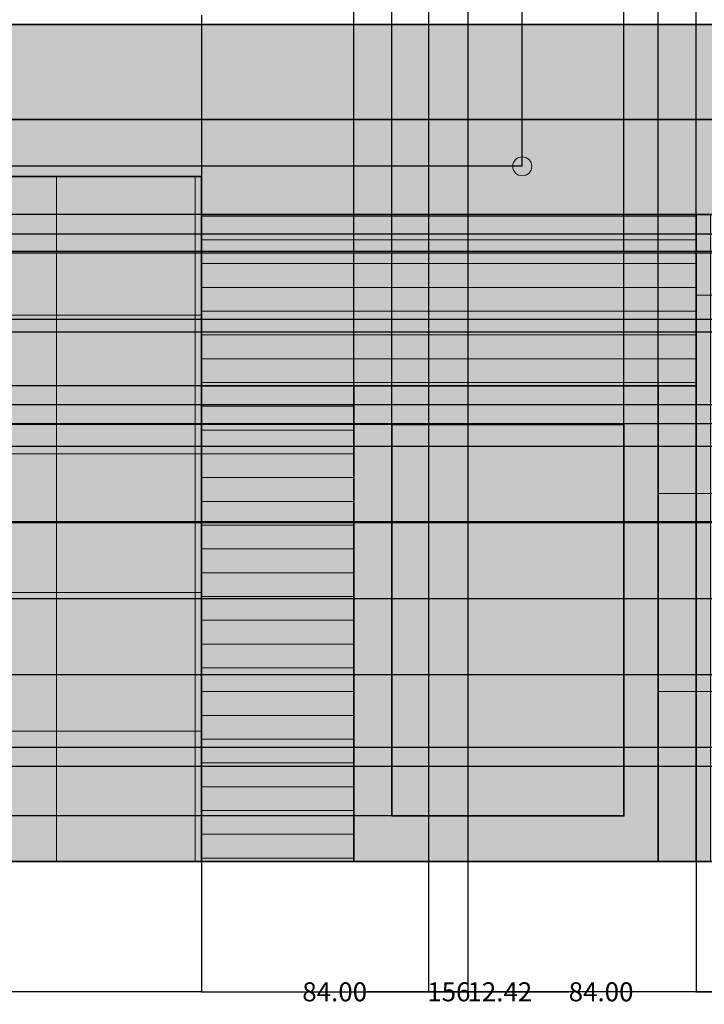
# Model space of a CAD drawing. Units: inches. Extents: x 148 to 1080, y 89 to 707.
# Tile 7 of 12: x 470 to 686, y 89 to 399. Entities that reach past the tile are written whole.
import ezdxf

# ---------------------------------------------------------------- set-up
doc = ezdxf.new("R2010")
doc.units = ezdxf.units.IN
doc.header["$MEASUREMENT"] = 0
for name, color, linetype, lineweight in [('A-ANNO-DIMS', 2, 'Continuous', 18), ('A-ELEV', 7, 'Continuous', 35), ('A-ELEV-PATT', 8, 'Continuous', 13), ('E-LITE', 3, 'Continuous', 18)]:
    doc.layers.add(name, color=color, linetype=linetype, lineweight=lineweight)
doc.styles.get("Standard").update_dxf_attribs({"font": 'arial.ttf'})
doc.dimstyles.get("Standard").update_dxf_attribs({"dimtxt": 6, "dimasz": 0.18, "dimexe": 0.18, "dimexo": 0.0625, "dimgap": 0.09, "dimtad": 0, "dimtih": 1, "dimtoh": 1, "dimdec": 0, "dimzin": 0, "dimdsep": 46, "dimlunit": 3, "dimtxsty": 'Standard', "dimcen": 0.09, "dimadec": 0, "dimazin": 0, "dimtfac": 1, "dimtdec": 0, "dimtofl": 0, "dimtmove": 0, "dimatfit": 3, "dimfxl": 1, "dimtolj": 1, "dimtzin": 0, "dimarcsym": 0})

# ---------------------------------------------------------------- blocks, each defined once
blk = doc.blocks.new('*D1')
at = {"layer": 'A-ANNO-DIMS', "color": 0, "lineweight": -2, "transparency": 16777216}
for p, q in [((215.02, 662.01), (215.02, 703.28)), ((215.2, 703.1), (604.32, 703.1)), ((1006.77, 703.1), (617.65, 703.1)), ((1006.95, 338.01), (1006.95, 703.28))]:
    blk.add_line(p, q, dxfattribs=at)
at = {"layer": 'A-ANNO-DIMS', "color": 0, "transparency": 16777216}
for points in [[(215.2, 703.13), (215.2, 703.07), (215.02, 703.1)], [(1006.77, 703.13), (1006.77, 703.07), (1006.95, 703.1)]]:
    blk.add_solid(points, dxfattribs=at)
at = {"layer": 'Defpoints', "color": 0, "transparency": 16777216}
for p in [(1006.95, 703.1), (215.02, 661.95), (1006.95, 337.95)]:
    blk.add_point(p, dxfattribs=at)
at = {"layer": 'A-ANNO-DIMS', "color": 0, "transparency": 16777216, "insert": (610.98, 703.1), "char_height": 6, "attachment_point": 5}
blk.add_mtext('\\A1;792', dxfattribs=at)
blk = doc.blocks.new('*D2')
at = {"layer": 'A-ANNO-DIMS', "color": 0, "lineweight": -2, "transparency": 16777216}
for p, q in [((251.02, 133.88), (251.02, 92.62)), ((527.02, 133.88), (527.02, 92.62)), ((251.2, 92.8), (382.25, 92.8)), ((526.84, 92.8), (395.79, 92.8))]:
    blk.add_line(p, q, dxfattribs=at)
at = {"layer": 'A-ANNO-DIMS', "color": 0, "transparency": 16777216}
for points in [[(251.2, 92.83), (251.2, 92.77), (251.02, 92.8)], [(526.84, 92.83), (526.84, 92.77), (527.02, 92.8)]]:
    blk.add_solid(points, dxfattribs=at)
at = {"layer": 'Defpoints', "color": 0, "transparency": 16777216}
for p in [(251.02, 133.95), (527.02, 133.95), (527.02, 92.8)]:
    blk.add_point(p, dxfattribs=at)
at = {"layer": 'A-ANNO-DIMS', "color": 0, "transparency": 16777216, "insert": (389.02, 92.8), "char_height": 6, "attachment_point": 5}
blk.add_mtext('\\A1;276', dxfattribs=at)
blk = doc.blocks.new('*D3')
at = {"layer": 'A-ANNO-DIMS', "color": 0, "lineweight": -2, "transparency": 16777216}
for p, q in [((527.02, 133.88), (527.02, 92.62)), ((683.02, 133.88), (683.02, 92.62)), ((527.2, 92.8), (598.59, 92.8)), ((682.84, 92.8), (611.45, 92.8))]:
    blk.add_line(p, q, dxfattribs=at)
at = {"layer": 'A-ANNO-DIMS', "color": 0, "transparency": 16777216}
for points in [[(527.2, 92.83), (527.2, 92.77), (527.02, 92.8)], [(682.84, 92.83), (682.84, 92.77), (683.02, 92.8)]]:
    blk.add_solid(points, dxfattribs=at)
at = {"layer": 'Defpoints', "color": 0, "transparency": 16777216}
for p in [(527.02, 133.95), (683.02, 133.95), (683.02, 92.8)]:
    blk.add_point(p, dxfattribs=at)
at = {"layer": 'A-ANNO-DIMS', "color": 0, "transparency": 16777216, "insert": (605.02, 92.8), "char_height": 6, "attachment_point": 5}
blk.add_mtext('\\A1;156', dxfattribs=at)
blk = doc.blocks.new('*D4')
at = {"layer": 'A-ANNO-DIMS', "color": 0, "lineweight": -2, "transparency": 16777216}
for p, q in [((683.02, 133.88), (683.02, 92.62)), ((719.02, 133.88), (719.02, 92.62)), ((683.2, 92.8), (696.64, 92.8)), ((718.84, 92.8), (705.4, 92.8))]:
    blk.add_line(p, q, dxfattribs=at)
at = {"layer": 'A-ANNO-DIMS', "color": 0, "transparency": 16777216}
for points in [[(683.2, 92.83), (683.2, 92.77), (683.02, 92.8)], [(718.84, 92.83), (718.84, 92.77), (719.02, 92.8)]]:
    blk.add_solid(points, dxfattribs=at)
at = {"layer": 'Defpoints', "color": 0, "transparency": 16777216}
for p in [(683.02, 133.95), (719.02, 133.95), (719.02, 92.8)]:
    blk.add_point(p, dxfattribs=at)
at = {"layer": 'A-ANNO-DIMS', "color": 0, "transparency": 16777216, "insert": (701.02, 92.8), "char_height": 6, "attachment_point": 5}
blk.add_mtext('\\A1;36', dxfattribs=at)
blk = doc.blocks.new('*D18')
at = {"layer": 'A-ANNO-DIMS', "color": 0, "lineweight": -2, "transparency": 16777216}
for p, q in [((635.08, 661.95), (1064.5, 661.95)), ((1064.32, 661.77), (1064.32, 401.1)), ((1064.32, 134.13), (1064.32, 394.79)), ((1007.01, 133.95), (1064.5, 133.95))]:
    blk.add_line(p, q, dxfattribs=at)
at = {"layer": 'A-ANNO-DIMS', "color": 0, "transparency": 16777216}
for points in [[(1064.29, 661.77), (1064.35, 661.77), (1064.32, 661.95)], [(1064.29, 134.13), (1064.35, 134.13), (1064.32, 133.95)]]:
    blk.add_solid(points, dxfattribs=at)
at = {"layer": 'Defpoints', "color": 0, "transparency": 16777216}
for p in [(635.02, 661.95), (1064.32, 661.95), (1006.95, 133.95)]:
    blk.add_point(p, dxfattribs=at)
at = {"layer": 'A-ANNO-DIMS', "color": 0, "transparency": 16777216, "insert": (1064.32, 397.95), "char_height": 6, "attachment_point": 5}
blk.add_mtext('\\A1;528', dxfattribs=at)
blk = doc.blocks.new('*D31')
at = {"layer": 'A-ANNO-DIMS', "color": 0, "lineweight": -2, "transparency": 16777216}
for p, q in [((587.06, 271.84), (587.06, 703.28)), ((587.24, 703.1), (613.42, 703.1)), ((660.03, 703.1), (633.85, 703.1)), ((660.21, 271.84), (660.21, 703.28))]:
    blk.add_line(p, q, dxfattribs=at)
at = {"layer": 'A-ANNO-DIMS', "color": 0, "transparency": 16777216}
for points in [[(587.24, 703.13), (587.24, 703.07), (587.06, 703.1)], [(660.03, 703.13), (660.03, 703.07), (660.21, 703.1)]]:
    blk.add_solid(points, dxfattribs=at)
at = {"layer": 'Defpoints', "color": 0, "transparency": 16777216}
for p in [(660.21, 703.1), (587.06, 271.77), (660.21, 271.77)]:
    blk.add_point(p, dxfattribs=at)
at = {"layer": 'A-ANNO-DIMS', "color": 0, "transparency": 16777216, "insert": (623.64, 703.1), "char_height": 6, "attachment_point": 5}
blk.add_mtext('\\A1;73.15', dxfattribs=at)
blk = doc.blocks.new('*D32')
at = {"layer": 'A-ANNO-DIMS', "color": 0, "lineweight": -2, "transparency": 16777216}
for p, q in [((587, 271.77), (160.42, 271.77)), ((160.6, 271.59), (160.6, 213.18)), ((160.6, 148.46), (160.6, 206.87)), ((587, 148.28), (160.42, 148.28))]:
    blk.add_line(p, q, dxfattribs=at)
at = {"layer": 'A-ANNO-DIMS', "color": 0, "transparency": 16777216}
for points in [[(160.57, 271.59), (160.63, 271.59), (160.6, 271.77)], [(160.57, 148.46), (160.63, 148.46), (160.6, 148.28)]]:
    blk.add_solid(points, dxfattribs=at)
at = {"layer": 'Defpoints', "color": 0, "transparency": 16777216}
for p in [(160.6, 271.77), (587.06, 271.77), (587.06, 148.28)]:
    blk.add_point(p, dxfattribs=at)
at = {"layer": 'A-ANNO-DIMS', "color": 0, "transparency": 16777216, "insert": (160.6, 210.03), "char_height": 6, "attachment_point": 5}
blk.add_mtext('\\A1;123.5', dxfattribs=at)
blk = doc.blocks.new('*D33')
at = {"layer": 'A-ANNO-DIMS', "color": 0, "lineweight": -2, "transparency": 16777216}
for p, q in [((575.02, 284.01), (575.02, 703.28)), ((575.2, 703.1), (618.63, 703.1)), ((670.84, 703.1), (627.41, 703.1)), ((671.02, 284.01), (671.02, 703.28))]:
    blk.add_line(p, q, dxfattribs=at)
at = {"layer": 'A-ANNO-DIMS', "color": 0, "transparency": 16777216}
for points in [[(575.2, 703.13), (575.2, 703.07), (575.02, 703.1)], [(670.84, 703.13), (670.84, 703.07), (671.02, 703.1)]]:
    blk.add_solid(points, dxfattribs=at)
at = {"layer": 'Defpoints', "color": 0, "transparency": 16777216}
for p in [(671.02, 703.1), (575.02, 283.95), (671.02, 283.95)]:
    blk.add_point(p, dxfattribs=at)
at = {"layer": 'A-ANNO-DIMS', "color": 0, "transparency": 16777216, "insert": (623.02, 703.1), "char_height": 6, "attachment_point": 5}
blk.add_mtext('\\A1;96', dxfattribs=at)
blk = doc.blocks.new('*D34')
at = {"layer": 'A-ANNO-DIMS', "color": 0, "lineweight": -2, "transparency": 16777216}
for p, q in [((574.96, 283.95), (160.42, 283.95)), ((160.6, 283.77), (160.6, 212.1)), ((160.6, 134.13), (160.6, 205.79)), ((574.96, 133.95), (160.42, 133.95))]:
    blk.add_line(p, q, dxfattribs=at)
at = {"layer": 'A-ANNO-DIMS', "color": 0, "transparency": 16777216}
for points in [[(160.57, 283.77), (160.63, 283.77), (160.6, 283.95)], [(160.57, 134.13), (160.63, 134.13), (160.6, 133.95)]]:
    blk.add_solid(points, dxfattribs=at)
at = {"layer": 'Defpoints', "color": 0, "transparency": 16777216}
for p in [(575.02, 283.95), (160.6, 133.95), (575.02, 133.95)]:
    blk.add_point(p, dxfattribs=at)
at = {"layer": 'A-ANNO-DIMS', "color": 0, "transparency": 16777216, "insert": (160.6, 208.95), "char_height": 6, "attachment_point": 5}
blk.add_mtext('\\A1;150', dxfattribs=at)
blk = doc.blocks.new('*D38')
at = {"layer": 'A-ANNO-DIMS', "color": 0, "lineweight": -2, "transparency": 16777216}
for p, q in [((934.89, 271.95), (160.42, 271.95)), ((160.6, 271.77), (160.6, 206.1)), ((160.6, 134.13), (160.6, 199.79)), ((934.89, 133.95), (160.42, 133.95))]:
    blk.add_line(p, q, dxfattribs=at)
at = {"layer": 'A-ANNO-DIMS', "color": 0, "transparency": 16777216}
for points in [[(160.57, 271.77), (160.63, 271.77), (160.6, 271.95)], [(160.57, 134.13), (160.63, 134.13), (160.6, 133.95)]]:
    blk.add_solid(points, dxfattribs=at)
at = {"layer": 'Defpoints', "color": 0, "transparency": 16777216}
for p in [(934.95, 271.95), (160.6, 133.95), (934.95, 133.95)]:
    blk.add_point(p, dxfattribs=at)
at = {"layer": 'A-ANNO-DIMS', "color": 0, "transparency": 16777216, "insert": (160.6, 202.95), "char_height": 6, "attachment_point": 5}
blk.add_mtext('\\A1;138', dxfattribs=at)
blk = doc.blocks.new('*D39')
at = {"layer": 'A-ANNO-DIMS', "color": 0, "lineweight": -2, "transparency": 16777216}
for p, q in [((946.89, 337.95), (160.42, 337.95)), ((160.6, 337.77), (160.6, 311.1)), ((160.6, 278.13), (160.6, 304.79)), ((946.89, 277.95), (160.42, 277.95))]:
    blk.add_line(p, q, dxfattribs=at)
at = {"layer": 'A-ANNO-DIMS', "color": 0, "transparency": 16777216}
for points in [[(160.57, 337.77), (160.63, 337.77), (160.6, 337.95)], [(160.57, 278.13), (160.63, 278.13), (160.6, 277.95)]]:
    blk.add_solid(points, dxfattribs=at)
at = {"layer": 'Defpoints', "color": 0, "transparency": 16777216}
for p in [(160.6, 337.95), (946.95, 337.95), (946.95, 277.95)]:
    blk.add_point(p, dxfattribs=at)
at = {"layer": 'A-ANNO-DIMS', "color": 0, "transparency": 16777216, "insert": (160.6, 307.95), "char_height": 6, "attachment_point": 5}
blk.add_mtext('\\A1;60', dxfattribs=at)
blk = doc.blocks.new('*D42')
at = {"layer": 'A-ANNO-DIMS', "color": 0, "lineweight": -2, "transparency": 16777216}
for p, q in [((772.96, 367.95), (160.42, 367.95)), ((160.6, 367.77), (160.6, 350.31)), ((160.6, 326.54), (160.6, 344)), ((718.96, 326.36), (160.42, 326.36))]:
    blk.add_line(p, q, dxfattribs=at)
at = {"layer": 'A-ANNO-DIMS', "color": 0, "transparency": 16777216}
for points in [[(160.57, 367.77), (160.63, 367.77), (160.6, 367.95)], [(160.57, 326.54), (160.63, 326.54), (160.6, 326.36)]]:
    blk.add_solid(points, dxfattribs=at)
at = {"layer": 'Defpoints', "color": 0, "transparency": 16777216}
for p in [(773.02, 367.95), (160.6, 326.36), (719.02, 326.36)]:
    blk.add_point(p, dxfattribs=at)
at = {"layer": 'A-ANNO-DIMS', "color": 0, "transparency": 16777216, "insert": (160.6, 347.16), "char_height": 6, "attachment_point": 5}
blk.add_mtext('\\A1;41.584', dxfattribs=at)
blk = doc.blocks.new('*D43')
at = {"layer": 'A-ANNO-DIMS', "color": 0, "lineweight": -2, "transparency": 16777216}
for p, q in [((765.88, 241.1), (160.42, 241.1)), ((160.6, 240.92), (160.6, 190.68)), ((160.6, 134.13), (160.6, 184.37)), ((776.65, 133.95), (160.42, 133.95))]:
    blk.add_line(p, q, dxfattribs=at)
at = {"layer": 'A-ANNO-DIMS', "color": 0, "transparency": 16777216}
for points in [[(160.57, 240.92), (160.63, 240.92), (160.6, 241.1)], [(160.57, 134.13), (160.63, 134.13), (160.6, 133.95)]]:
    blk.add_solid(points, dxfattribs=at)
at = {"layer": 'Defpoints', "color": 0, "transparency": 16777216}
for p in [(765.95, 241.1), (160.6, 133.95), (776.71, 133.95)]:
    blk.add_point(p, dxfattribs=at)
at = {"layer": 'A-ANNO-DIMS', "color": 0, "transparency": 16777216, "insert": (160.6, 187.52), "char_height": 6, "attachment_point": 5}
blk.add_mtext('\\A1;107.15', dxfattribs=at)
blk = doc.blocks.new('*D47')
at = {"layer": 'A-ANNO-DIMS', "color": 0, "lineweight": -2, "transparency": 16777216}
for p, q in [((628.17, 353.26), (628.17, 703.28)), ((628.35, 703.1), (645.36, 703.1)), ((682.84, 703.1), (665.83, 703.1)), ((683.02, 338.01), (683.02, 703.28))]:
    blk.add_line(p, q, dxfattribs=at)
at = {"layer": 'A-ANNO-DIMS', "color": 0, "transparency": 16777216}
for points in [[(628.35, 703.13), (628.35, 703.07), (628.17, 703.1)], [(682.84, 703.13), (682.84, 703.07), (683.02, 703.1)]]:
    blk.add_solid(points, dxfattribs=at)
at = {"layer": 'Defpoints', "color": 0, "transparency": 16777216}
for p in [(683.02, 703.1), (628.17, 353.2), (683.02, 337.95)]:
    blk.add_point(p, dxfattribs=at)
at = {"layer": 'A-ANNO-DIMS', "color": 0, "transparency": 16777216, "insert": (655.6, 703.1), "char_height": 6, "attachment_point": 5}
blk.add_mtext('\\A1;54.85', dxfattribs=at)
blk = doc.blocks.new('*D48')
at = {"layer": 'A-ANNO-DIMS', "color": 0, "lineweight": -2, "transparency": 16777216}
for p, q in [((683.02, 338.01), (683.02, 703.28)), ((683.2, 703.1), (694.68, 703.1)), ((726.76, 703.1), (715.28, 703.1)), ((726.94, 354.92), (726.94, 703.28))]:
    blk.add_line(p, q, dxfattribs=at)
at = {"layer": 'A-ANNO-DIMS', "color": 0, "transparency": 16777216}
for points in [[(683.2, 703.13), (683.2, 703.07), (683.02, 703.1)], [(726.76, 703.13), (726.76, 703.07), (726.94, 703.1)]]:
    blk.add_solid(points, dxfattribs=at)
at = {"layer": 'Defpoints', "color": 0, "transparency": 16777216}
for p in [(726.94, 703.1), (726.94, 354.86), (683.02, 337.95)]:
    blk.add_point(p, dxfattribs=at)
at = {"layer": 'A-ANNO-DIMS', "color": 0, "transparency": 16777216, "insert": (704.98, 703.1), "char_height": 6, "attachment_point": 5}
blk.add_mtext('\\A1;43.92', dxfattribs=at)
blk = doc.blocks.new('*D49')
at = {"layer": 'A-ANNO-DIMS', "color": 0, "lineweight": -2, "transparency": 16777216}
for p, q in [((628.11, 353.2), (160.42, 353.2)), ((160.6, 353.02), (160.6, 348.73)), ((160.6, 338.13), (160.6, 342.42)), ((682.96, 337.95), (160.42, 337.95))]:
    blk.add_line(p, q, dxfattribs=at)
at = {"layer": 'A-ANNO-DIMS', "color": 0, "transparency": 16777216}
for points in [[(160.57, 353.02), (160.63, 353.02), (160.6, 353.2)], [(160.57, 338.13), (160.63, 338.13), (160.6, 337.95)]]:
    blk.add_solid(points, dxfattribs=at)
at = {"layer": 'Defpoints', "color": 0, "transparency": 16777216}
for p in [(628.17, 353.2), (160.6, 337.95), (683.02, 337.95)]:
    blk.add_point(p, dxfattribs=at)
at = {"layer": 'A-ANNO-DIMS', "color": 0, "transparency": 16777216, "insert": (160.6, 345.57), "char_height": 6, "attachment_point": 5}
blk.add_mtext('\\A1;15.248', dxfattribs=at)
blk = doc.blocks.new('*D50')
at = {"layer": 'A-ANNO-DIMS', "color": 0, "lineweight": -2, "transparency": 16777216}
for p, q in [((727, 354.86), (1064.5, 354.86)), ((1064.32, 354.68), (1064.32, 349.56)), ((1064.32, 338.13), (1064.32, 343.25)), ((683.08, 337.95), (1064.5, 337.95))]:
    blk.add_line(p, q, dxfattribs=at)
at = {"layer": 'A-ANNO-DIMS', "color": 0, "transparency": 16777216}
for points in [[(1064.29, 354.68), (1064.35, 354.68), (1064.32, 354.86)], [(1064.29, 338.13), (1064.35, 338.13), (1064.32, 337.95)]]:
    blk.add_solid(points, dxfattribs=at)
at = {"layer": 'Defpoints', "color": 0, "transparency": 16777216}
for p in [(726.94, 354.86), (683.02, 337.95), (1064.32, 337.95)]:
    blk.add_point(p, dxfattribs=at)
at = {"layer": 'A-ANNO-DIMS', "color": 0, "transparency": 16777216, "insert": (1064.32, 346.4), "char_height": 6, "attachment_point": 5}
blk.add_mtext('\\A1;16.912', dxfattribs=at)
blk = doc.blocks.new('*D55')
at = {"layer": 'A-ANNO-DIMS', "color": 0, "lineweight": -2, "transparency": 16777216}
for p, q in [((598.6, 541.88), (598.6, 92.62)), ((611.02, 541.88), (611.02, 92.62)), ((598.78, 92.8), (610.84, 92.8)), ((611.02, 92.8), (611.2, 92.8))]:
    blk.add_line(p, q, dxfattribs=at)
at = {"layer": 'A-ANNO-DIMS', "color": 0, "transparency": 16777216}
for points in [[(598.78, 92.83), (598.78, 92.77), (598.6, 92.8)], [(610.84, 92.83), (610.84, 92.77), (611.02, 92.8)]]:
    blk.add_solid(points, dxfattribs=at)
at = {"layer": 'Defpoints', "color": 0, "transparency": 16777216}
for p in [(598.6, 541.95), (611.02, 541.95), (611.02, 92.8)]:
    blk.add_point(p, dxfattribs=at)
at = {"layer": 'A-ANNO-DIMS', "color": 0, "transparency": 16777216, "insert": (621.1, 92.8), "char_height": 6, "attachment_point": 5}
blk.add_mtext('\\A1;12.42', dxfattribs=at)
blk = doc.blocks.new('*D57')
at = {"layer": 'A-ANNO-DIMS', "color": 0, "lineweight": -2, "transparency": 16777216}
for p, q in [((527.02, 400.88), (527.02, 92.62)), ((611.02, 400.88), (611.02, 92.62)), ((527.2, 92.8), (558.81, 92.8)), ((610.84, 92.8), (579.23, 92.8))]:
    blk.add_line(p, q, dxfattribs=at)
at = {"layer": 'A-ANNO-DIMS', "color": 0, "transparency": 16777216}
for points in [[(527.2, 92.83), (527.2, 92.77), (527.02, 92.8)], [(610.84, 92.83), (610.84, 92.77), (611.02, 92.8)]]:
    blk.add_solid(points, dxfattribs=at)
at = {"layer": 'Defpoints', "color": 0, "transparency": 16777216}
for p in [(527.02, 400.95), (611.02, 400.95), (611.02, 92.8)]:
    blk.add_point(p, dxfattribs=at)
at = {"layer": 'A-ANNO-DIMS', "color": 0, "transparency": 16777216, "insert": (569.02, 92.8), "char_height": 6, "attachment_point": 5}
blk.add_mtext('\\A1;84.00', dxfattribs=at)
blk = doc.blocks.new('*D58')
at = {"layer": 'A-ANNO-DIMS', "color": 0, "lineweight": -2, "transparency": 16777216}
for p, q in [((611.02, 400.88), (611.02, 92.62)), ((695.02, 400.88), (695.02, 92.62)), ((611.2, 92.8), (642.81, 92.8)), ((694.84, 92.8), (663.23, 92.8))]:
    blk.add_line(p, q, dxfattribs=at)
at = {"layer": 'A-ANNO-DIMS', "color": 0, "transparency": 16777216}
for points in [[(611.2, 92.83), (611.2, 92.77), (611.02, 92.8)], [(694.84, 92.83), (694.84, 92.77), (695.02, 92.8)]]:
    blk.add_solid(points, dxfattribs=at)
at = {"layer": 'Defpoints', "color": 0, "transparency": 16777216}
for p in [(611.02, 400.95), (695.02, 400.95), (695.02, 92.8)]:
    blk.add_point(p, dxfattribs=at)
at = {"layer": 'A-ANNO-DIMS', "color": 0, "transparency": 16777216, "insert": (653.02, 92.8), "char_height": 6, "attachment_point": 5}
blk.add_mtext('\\A1;84.00', dxfattribs=at)
blk = doc.blocks.new('*D71')
at = {"layer": 'A-ANNO-DIMS', "color": 0, "lineweight": -2, "transparency": 16777216}
for p, q in [((389.08, 169.95), (1064.5, 169.95)), ((1064.32, 169.95), (1064.32, 170.13)), ((1064.32, 170.13), (1064.5, 170.13)), ((1064.32, 164.13), (1064.32, 169.77)), ((395.08, 163.95), (1064.5, 163.95))]:
    blk.add_line(p, q, dxfattribs=at)
at = {"layer": 'A-ANNO-DIMS', "color": 0, "transparency": 16777216}
for points in [[(1064.29, 169.77), (1064.35, 169.77), (1064.32, 169.95)], [(1064.29, 164.13), (1064.35, 164.13), (1064.32, 163.95)]]:
    blk.add_solid(points, dxfattribs=at)
at = {"layer": 'Defpoints', "color": 0, "transparency": 16777216}
for p in [(389.02, 169.95), (1064.32, 169.95), (395.02, 163.95)]:
    blk.add_point(p, dxfattribs=at)
at = {"layer": 'A-ANNO-DIMS', "color": 0, "transparency": 16777216, "insert": (1072.39, 170.13), "char_height": 6, "attachment_point": 5}
blk.add_mtext('\\A1;6.00', dxfattribs=at)
blk = doc.blocks.new('*D72')
at = {"layer": 'A-ANNO-DIMS', "color": 0, "lineweight": -2, "transparency": 16777216}
for p, q in [((389.08, 192.87), (1064.5, 192.87)), ((1064.32, 192.69), (1064.32, 184.56)), ((1064.32, 170.13), (1064.32, 178.26)), ((389.08, 169.95), (1064.5, 169.95))]:
    blk.add_line(p, q, dxfattribs=at)
at = {"layer": 'A-ANNO-DIMS', "color": 0, "transparency": 16777216}
for points in [[(1064.29, 192.69), (1064.35, 192.69), (1064.32, 192.87)], [(1064.29, 170.13), (1064.35, 170.13), (1064.32, 169.95)]]:
    blk.add_solid(points, dxfattribs=at)
at = {"layer": 'Defpoints', "color": 0, "transparency": 16777216}
for p in [(389.02, 192.87), (1064.32, 192.87), (389.02, 169.95)]:
    blk.add_point(p, dxfattribs=at)
at = {"layer": 'A-ANNO-DIMS', "color": 0, "transparency": 16777216, "insert": (1064.32, 181.41), "char_height": 6, "attachment_point": 5}
blk.add_mtext('\\A1;22.92', dxfattribs=at)
blk = doc.blocks.new('*D73')
at = {"layer": 'A-ANNO-DIMS', "color": 0, "lineweight": -2, "transparency": 16777216}
for p, q in [((389.08, 216.87), (1064.5, 216.87)), ((1064.32, 216.69), (1064.32, 208.02)), ((1064.32, 193.05), (1064.32, 201.72)), ((389.08, 192.87), (1064.5, 192.87))]:
    blk.add_line(p, q, dxfattribs=at)
at = {"layer": 'A-ANNO-DIMS', "color": 0, "transparency": 16777216}
for points in [[(1064.29, 216.69), (1064.35, 216.69), (1064.32, 216.87)], [(1064.29, 193.05), (1064.35, 193.05), (1064.32, 192.87)]]:
    blk.add_solid(points, dxfattribs=at)
at = {"layer": 'Defpoints', "color": 0, "transparency": 16777216}
for p in [(389.02, 216.87), (1064.32, 216.87), (389.02, 192.87)]:
    blk.add_point(p, dxfattribs=at)
at = {"layer": 'A-ANNO-DIMS', "color": 0, "transparency": 16777216, "insert": (1064.32, 204.87), "char_height": 6, "attachment_point": 5}
blk.add_mtext('\\A1;24.00', dxfattribs=at)
blk = doc.blocks.new('*D74')
at = {"layer": 'A-ANNO-DIMS', "color": 0, "lineweight": -2, "transparency": 16777216}
for p, q in [((389.08, 240.87), (1064.5, 240.87)), ((1064.32, 240.69), (1064.32, 232.02)), ((1064.32, 217.05), (1064.32, 225.72)), ((389.08, 216.87), (1064.5, 216.87))]:
    blk.add_line(p, q, dxfattribs=at)
at = {"layer": 'A-ANNO-DIMS', "color": 0, "transparency": 16777216}
for points in [[(1064.29, 240.69), (1064.35, 240.69), (1064.32, 240.87)], [(1064.29, 217.05), (1064.35, 217.05), (1064.32, 216.87)]]:
    blk.add_solid(points, dxfattribs=at)
at = {"layer": 'Defpoints', "color": 0, "transparency": 16777216}
for p in [(389.02, 240.87), (1064.32, 240.87), (389.02, 216.87)]:
    blk.add_point(p, dxfattribs=at)
at = {"layer": 'A-ANNO-DIMS', "color": 0, "transparency": 16777216, "insert": (1064.32, 228.87), "char_height": 6, "attachment_point": 5}
blk.add_mtext('\\A1;24.00', dxfattribs=at)
blk = doc.blocks.new('*D75')
at = {"layer": 'A-ANNO-DIMS', "color": 0, "lineweight": -2, "transparency": 16777216}
for p, q in [((389.08, 264.87), (1064.5, 264.87)), ((1064.32, 264.69), (1064.32, 256.02)), ((1064.32, 241.05), (1064.32, 249.72)), ((389.08, 240.87), (1064.5, 240.87))]:
    blk.add_line(p, q, dxfattribs=at)
at = {"layer": 'A-ANNO-DIMS', "color": 0, "transparency": 16777216}
for points in [[(1064.29, 264.69), (1064.35, 264.69), (1064.32, 264.87)], [(1064.29, 241.05), (1064.35, 241.05), (1064.32, 240.87)]]:
    blk.add_solid(points, dxfattribs=at)
at = {"layer": 'Defpoints', "color": 0, "transparency": 16777216}
for p in [(389.02, 264.87), (1064.32, 264.87), (389.02, 240.87)]:
    blk.add_point(p, dxfattribs=at)
at = {"layer": 'A-ANNO-DIMS', "color": 0, "transparency": 16777216, "insert": (1064.32, 252.87), "char_height": 6, "attachment_point": 5}
blk.add_mtext('\\A1;24.00', dxfattribs=at)
blk = doc.blocks.new('*D76')
at = {"layer": 'A-ANNO-DIMS', "color": 0, "lineweight": -2, "transparency": 16777216}
for p, q in [((389.08, 300.95), (1064.5, 300.95)), ((1064.32, 300.77), (1064.32, 286.06)), ((1064.32, 265.05), (1064.32, 279.75)), ((389.08, 264.87), (1064.5, 264.87))]:
    blk.add_line(p, q, dxfattribs=at)
at = {"layer": 'A-ANNO-DIMS', "color": 0, "transparency": 16777216}
for points in [[(1064.29, 300.77), (1064.35, 300.77), (1064.32, 300.95)], [(1064.29, 265.05), (1064.35, 265.05), (1064.32, 264.87)]]:
    blk.add_solid(points, dxfattribs=at)
at = {"layer": 'Defpoints', "color": 0, "transparency": 16777216}
for p in [(389.02, 300.95), (1064.32, 300.95), (389.02, 264.87)]:
    blk.add_point(p, dxfattribs=at)
at = {"layer": 'A-ANNO-DIMS', "color": 0, "transparency": 16777216, "insert": (1064.32, 282.91), "char_height": 6, "attachment_point": 5}
blk.add_mtext('\\A1;36.08', dxfattribs=at)
blk = doc.blocks.new('*D77')
at = {"layer": 'A-ANNO-DIMS', "color": 0, "lineweight": -2, "transparency": 16777216}
for p, q in [((389.08, 304.95), (1064.5, 304.95)), ((1064.32, 304.95), (1064.32, 305.13)), ((1064.32, 305.13), (1064.5, 305.13)), ((1064.32, 301.13), (1064.32, 304.77)), ((389.08, 300.95), (1064.5, 300.95))]:
    blk.add_line(p, q, dxfattribs=at)
at = {"layer": 'A-ANNO-DIMS', "color": 0, "transparency": 16777216}
for points in [[(1064.29, 304.77), (1064.35, 304.77), (1064.32, 304.95)], [(1064.29, 301.13), (1064.35, 301.13), (1064.32, 300.95)]]:
    blk.add_solid(points, dxfattribs=at)
at = {"layer": 'Defpoints', "color": 0, "transparency": 16777216}
for p in [(389.02, 304.95), (1064.32, 304.95), (389.02, 300.95)]:
    blk.add_point(p, dxfattribs=at)
at = {"layer": 'A-ANNO-DIMS', "color": 0, "transparency": 16777216, "insert": (1072.5, 305.13), "char_height": 6, "attachment_point": 5}
blk.add_mtext('\\A1;4.00', dxfattribs=at)
blk = doc.blocks.new('*D78')
at = {"layer": 'A-ANNO-DIMS', "color": 0, "lineweight": -2, "transparency": 16777216}
for p, q in [((389.08, 325.95), (1064.5, 325.95)), ((1064.32, 325.77), (1064.32, 318.6)), ((1064.32, 305.13), (1064.32, 312.29)), ((389.08, 304.95), (1064.5, 304.95))]:
    blk.add_line(p, q, dxfattribs=at)
at = {"layer": 'A-ANNO-DIMS', "color": 0, "transparency": 16777216}
for points in [[(1064.29, 325.77), (1064.35, 325.77), (1064.32, 325.95)], [(1064.29, 305.13), (1064.35, 305.13), (1064.32, 304.95)]]:
    blk.add_solid(points, dxfattribs=at)
at = {"layer": 'Defpoints', "color": 0, "transparency": 16777216}
for p in [(389.02, 325.95), (1064.32, 325.95), (389.02, 304.95)]:
    blk.add_point(p, dxfattribs=at)
at = {"layer": 'A-ANNO-DIMS', "color": 0, "transparency": 16777216, "insert": (1064.32, 315.45), "char_height": 6, "attachment_point": 5}
blk.add_mtext('\\A1;21.00', dxfattribs=at)
blk = doc.blocks.new('*D79')
at = {"layer": 'A-ANNO-DIMS', "color": 0, "lineweight": -2, "transparency": 16777216}
for p, q in [((395.08, 331.95), (1064.5, 331.95)), ((1064.32, 331.95), (1064.32, 332.13)), ((1064.32, 332.13), (1064.5, 332.13)), ((1064.32, 326.13), (1064.32, 331.77)), ((389.08, 325.95), (1064.5, 325.95))]:
    blk.add_line(p, q, dxfattribs=at)
at = {"layer": 'A-ANNO-DIMS', "color": 0, "transparency": 16777216}
for points in [[(1064.29, 331.77), (1064.35, 331.77), (1064.32, 331.95)], [(1064.29, 326.13), (1064.35, 326.13), (1064.32, 325.95)]]:
    blk.add_solid(points, dxfattribs=at)
at = {"layer": 'Defpoints', "color": 0, "transparency": 16777216}
for p in [(395.02, 331.95), (1064.32, 331.95), (389.02, 325.95)]:
    blk.add_point(p, dxfattribs=at)
at = {"layer": 'A-ANNO-DIMS', "color": 0, "transparency": 16777216, "insert": (1072.39, 332.13), "char_height": 6, "attachment_point": 5}
blk.add_mtext('\\A1;6.00', dxfattribs=at)
blk = doc.blocks.new('*D102')
at = {"layer": 'A-ANNO-DIMS', "color": 0, "lineweight": -2, "transparency": 16777216}
for p, q in [((742.96, 271.95), (160.42, 271.95)), ((160.6, 271.77), (160.6, 259.68)), ((160.6, 241.28), (160.6, 253.37)), ((765.88, 241.1), (160.42, 241.1))]:
    blk.add_line(p, q, dxfattribs=at)
at = {"layer": 'A-ANNO-DIMS', "color": 0, "transparency": 16777216}
for points in [[(160.57, 271.77), (160.63, 271.77), (160.6, 271.95)], [(160.57, 241.28), (160.63, 241.28), (160.6, 241.1)]]:
    blk.add_solid(points, dxfattribs=at)
at = {"layer": 'Defpoints', "color": 0, "transparency": 16777216}
for p in [(160.6, 271.95), (743.02, 271.95), (765.95, 241.1)]:
    blk.add_point(p, dxfattribs=at)
at = {"layer": 'A-ANNO-DIMS', "color": 0, "transparency": 16777216, "insert": (160.6, 256.52), "char_height": 6, "attachment_point": 5}
blk.add_mtext('\\A1;30.85', dxfattribs=at)

msp = doc.modelspace()

# ---------------------------------------------------------------- hatches: boundary and pattern name
at = {"layer": 'A-ELEV-PATT'}
h = msp.add_hatch(color=256, dxfattribs=at)
h.dxf.hatch_style = 1
h.paths.add_polyline_path([(635.0199, 661.9474), (611.0199, 661.9474), (215.0199, 661.9474), (215.0199, 631.9474), (611.0199, 631.9474), (635.0199, 631.9474)])
h.paths.add_polyline_path([(773.0199, 397.9474), (215.0199, 397.9474), (215.0199, 367.9474), (773.0199, 367.9474)])
h = msp.add_hatch(color=256, dxfattribs=at)
h.dxf.hatch_style = 1
h.paths.add_polyline_path([(622.6005, 631.9474), (611.0199, 631.9474), (215.0199, 631.9474), (251.0199, 542.9352), (251.0199, 601.9474), (527.0199, 601.9474), (527.0199, 541.9474), (598.6005, 541.9474)])
h.paths.add_polyline_path([(558.5775, 608.9493, -1), (552.5775, 608.9493, -1)], flags=16)
h.paths.add_polyline_path([(586.7589, 556.0652, -1), (580.7589, 556.0652, -1)], flags=16)
h.paths.add_polyline_path([(635.0199, 631.9474), (622.6005, 631.9474), (598.6005, 541.9474), (611.0199, 541.9474)])
h.paths.add_polyline_path([(773.0199, 367.9474), (215.0199, 367.9474), (251.0199, 337.9474), (251.0199, 349.9474), (527.0199, 349.9474), (527.0199, 337.9474), (734.0628, 337.9474)])
h.paths.add_polyline_path([(631.1736, 353.1958, -1), (625.1736, 353.1958, -1)], flags=16)
h.paths.add_polyline_path([(729.9419, 354.8591, -1), (723.9419, 354.8591, -1)], flags=16)
h = msp.add_hatch(color=256, dxfattribs=at)
h.dxf.hatch_style = 1
h.paths.add_polyline_path([(552.5775, 608.9493, 1), (558.5775, 608.9493, 1)])
h.paths.add_polyline_path([(586.7589, 556.0652, 1), (580.7589, 556.0652, 1)])
h.paths.add_polyline_path([(625.1736, 353.1958, 1), (631.1736, 353.1958, 1)])
h.paths.add_polyline_path([(723.9419, 354.8591, 1), (729.9419, 354.8591, 1)])
h = msp.add_hatch(dxfattribs=at)
h.set_pattern_fill('ANSI31', color=256, scale=60, angle=135)
h.paths.add_polyline_path([(479.0199, 601.9474), (395.0199, 601.9474), (395.0199, 513.7706), (479.0199, 513.7706)])
h.paths.add_polyline_path([(479.0199, 513.7706), (395.0199, 513.7706), (395.0199, 400.9474), (479.0199, 400.9474)])
h.paths.add_polyline_path([(683.0199, 337.9474), (527.0199, 337.9474), (527.0199, 283.9474), (683.0199, 283.9474)])
h = msp.add_hatch(color=256, dxfattribs=at)
h.dxf.hatch_style = 1
h.paths.add_polyline_path([(527.0199, 349.9474), (395.0199, 349.9474), (395.0199, 271.2774), (527.0199, 272.3839)])
h.paths.add_polyline_path([(275.0199, 349.9474), (251.0199, 349.9474), (251.0199, 270.0704), (275.0199, 270.2716)])
h.paths.add_polyline_path([(743.0199, 337.9474), (734.0628, 337.9474), (719.0199, 326.3632), (719.0199, 277.9474), (743.0199, 277.9474)])
h.paths.add_polyline_path([(743.0199, 277.9474), (719.0199, 277.9474), (719.0199, 133.9474), (743.0199, 133.9474)])
h.paths.add_polyline_path([(734.0628, 337.9474), (719.0199, 337.9474), (719.0199, 326.3632)])
h = msp.add_hatch(dxfattribs=at)
h.set_pattern_fill('ANSI37', color=256, scale=350, angle=135)
h.paths.add_polyline_path([(527.0199, 349.9474), (395.0199, 349.9474), (395.0199, 163.9474), (275.0199, 163.9474), (275.0199, 349.9474), (251.0199, 349.9474), (251.0199, 133.9474), (527.0199, 133.9474)])
h = msp.add_hatch(color=256, dxfattribs=at)
h.dxf.hatch_style = 1
h.paths.add_polyline_path([(527.0199, 272.3839), (395.0199, 271.2774), (395.0199, 163.9474), (275.0199, 163.9474), (275.0199, 270.2716), (251.0199, 270.0704), (251.0199, 133.9474), (527.0199, 133.9474)])
h.paths.add_polyline_path([(1006.9492, 337.9474), (946.9492, 337.9474), (946.9492, 277.9474), (1006.9492, 277.9474)])
h.paths.add_polyline_path([(1006.9492, 277.9474), (946.9492, 277.9474), (946.9492, 133.9474), (1006.9492, 133.9474)])
h.paths.add_polyline_path([(946.9492, 337.9474), (743.0199, 337.9474), (743.0199, 277.9474), (946.9492, 277.9474)])
h = msp.add_hatch(color=256, dxfattribs=at)
h.dxf.hatch_style = 1
h.paths.add_polyline_path([(575.0199, 283.9474), (527.0199, 283.9474), (527.0199, 133.9474), (575.0199, 133.9474)])
h.paths.add_polyline_path([(683.0199, 337.9474), (527.0199, 337.9474), (527.0199, 283.9474), (683.0199, 283.9474)])
h = msp.add_hatch(dxfattribs=at)
h.set_pattern_fill('ANSI37', color=256, scale=500, angle=135)
h.paths.add_polyline_path([(946.9492, 337.9474), (743.0199, 337.9474), (743.0199, 277.9474), (946.9492, 277.9474)])
h.paths.add_polyline_path([(1006.9492, 337.9474), (946.9492, 337.9474), (946.9492, 277.9474), (1006.9492, 277.9474)])
h.paths.add_polyline_path([(1006.9492, 277.9474), (946.9492, 277.9474), (946.9492, 133.9474), (1006.9492, 133.9474)])
h.paths.add_polyline_path([(719.0199, 337.9474), (683.0199, 337.9474), (683.0199, 133.9474), (719.0199, 133.9474)])
h.paths.add_polyline_path([(743.0199, 277.9474), (719.0199, 277.9474), (719.0199, 133.9474), (743.0199, 133.9474)])
h.paths.add_polyline_path([(743.0199, 337.9474), (734.0628, 337.9474), (719.0199, 326.3632), (719.0199, 277.9474), (743.0199, 277.9474)])
h.paths.add_polyline_path([(683.0199, 283.9474), (671.0199, 283.9474), (671.0199, 133.9474), (683.0199, 133.9474)])
h = msp.add_hatch(color=256, dxfattribs=at)
h.dxf.hatch_style = 1
h.paths.add_polyline_path([(719.0199, 337.9474), (683.0199, 337.9474), (683.0199, 133.9474), (719.0199, 133.9474)])
h = msp.add_hatch(dxfattribs=at)
h.set_pattern_fill('ANSI31', color=256, scale=60, angle=135)
h.paths.add_polyline_path([(575.0199, 283.9474), (527.0199, 283.9474), (527.0199, 133.9474), (575.0199, 133.9474)])
h = msp.add_hatch(color=256, dxfattribs=at)
h.dxf.hatch_style = 1
h.paths.add_polyline_path([(660.2092, 271.7747), (587.0631, 271.7747), (587.0631, 148.2809), (660.2092, 148.2809)], flags=0)
h.paths.add_polyline_path([(671.0199, 283.9474), (575.0199, 283.9474), (575.0199, 133.9474), (671.0199, 133.9474)])
h.paths.add_polyline_path([(587.0631, 271.7747), (660.2092, 271.7747), (660.2092, 148.2809), (587.0631, 148.2809)], flags=16)
h = msp.add_hatch(color=256, dxfattribs=at)
h.dxf.hatch_style = 1
h.paths.add_polyline_path([(683.0199, 283.9474), (671.0199, 283.9474), (671.0199, 133.9474), (683.0199, 133.9474)])
h = msp.add_hatch(color=256, dxfattribs=at)
h.dxf.hatch_style = 1
h.paths.add_polyline_path([(660.2092, 271.7747), (587.0631, 271.7747), (587.0631, 148.2809), (660.2092, 148.2809)])

# ---------------------------------------------------------------- linework, layer by layer
at = {"layer": 'A-ELEV'}
for p, q in [((215.0199, 397.9474), (773.0199, 397.9474)), ((215.0199, 367.9474), (773.0199, 367.9474)), ((251.0199, 349.9474), (527.0199, 349.9474)), ((527.0199, 133.9474), (527.0199, 349.9474)), ((527.0199, 337.9474), (1006.9492, 337.9474)), ((683.0199, 133.9474), (683.0199, 337.9474)), ((527.0199, 283.9474), (683.0199, 283.9474)), ((575.0199, 133.9474), (575.0199, 283.9474)), ((671.0199, 133.9474), (671.0199, 283.9474)), ((201.7492, 133.9474), (1023.175, 133.9474))]:
    msp.add_line(p, q, dxfattribs=at)
msp.add_lwpolyline([(587.0631, 271.7747), (660.2092, 271.7747), (660.2092, 148.2809), (587.0631, 148.2809)], close=True, dxfattribs=at)
at = {"layer": 'E-LITE'}
msp.add_circle((628.1736, 353.1958), 3, dxfattribs=at)

# ---------------------------------------------------------------- dimensions: what is measured, and where the dimension line sits
at = {"layer": 'A-ANNO-DIMS'}
for base, p1, p2, override, picture, middle in [((1006.9492, 703.0974), (215.0199, 661.9474), (1006.9492, 337.9474), {"dimdec": 0, "dimlfac": 1, "dimrnd": 0, "dimzin": 0, "dimdsep": 46, "dimlunit": 2}, '*D1', (610.9845, 703.0974)), ((671.0199, 703.0974), (575.0199, 283.9474), (671.0199, 283.9474), {"dimdec": 0, "dimlfac": 1, "dimrnd": 0, "dimzin": 0, "dimdsep": 46, "dimlunit": 2}, '*D33', (623.0199, 703.0974)), ((660.2092, 703.0974), (587.0631, 271.7747), (660.2092, 271.7747), {"dimdec": 2, "dimlfac": 1, "dimrnd": 0, "dimzin": 0, "dimdsep": 46, "dimlunit": 2}, '*D31', (623.6362, 703.0974)), ((683.0199, 703.0974), (628.1736, 353.1958), (683.0199, 337.9474), {"dimdec": 2, "dimlfac": 1, "dimrnd": 0, "dimzin": 0, "dimdsep": 46, "dimlunit": 2}, '*D47', (655.5968, 703.0974)), ((726.9419, 703.0974), (683.0199, 337.9474), (726.9419, 354.8591), {"dimdec": 2, "dimlfac": 1, "dimrnd": 0, "dimzin": 0, "dimdsep": 46, "dimlunit": 2}, '*D48', (704.9809, 703.0974)), ((611.0199, 92.7974), (598.6005, 541.9474), (611.0199, 541.9474), {"dimdec": 2, "dimlfac": 1, "dimrnd": 0, "dimzin": 0, "dimdsep": 46, "dimlunit": 2}, '*D55', (621.1002, 92.7974)), ((611.0199, 92.7974), (527.0199, 400.9474), (611.0199, 400.9474), {"dimdec": 2, "dimlfac": 1, "dimrnd": 0, "dimzin": 0, "dimdsep": 46, "dimlunit": 2}, '*D57', (569.0199, 92.7974)), ((695.0199, 92.7974), (611.0199, 400.9474), (695.0199, 400.9474), {"dimdec": 2, "dimlfac": 1, "dimrnd": 0, "dimzin": 0, "dimdsep": 46, "dimlunit": 2}, '*D58', (653.0199, 92.7974)), ((527.0199, 92.7974), (251.0199, 133.9474), (527.0199, 133.9474), {"dimdec": 0, "dimlfac": 1, "dimrnd": 0, "dimzin": 0, "dimdsep": 46, "dimlunit": 2}, '*D2', (389.0199, 92.7974)), ((683.0199, 92.7974), (527.0199, 133.9474), (683.0199, 133.9474), {"dimdec": 0, "dimlfac": 1, "dimrnd": 0, "dimzin": 0, "dimdsep": 46, "dimlunit": 2}, '*D3', (605.0199, 92.7974)), ((719.0199, 92.7974), (683.0199, 133.9474), (719.0199, 133.9474), {"dimdec": 0, "dimlfac": 1, "dimrnd": 0, "dimzin": 0, "dimdsep": 46, "dimlunit": 2}, '*D4', (701.0199, 92.7974))]:
    dim = msp.add_linear_dim(base=base, p1=p1, p2=p2, dimstyle='Standard', override=override, dxfattribs=at)
    dim.commit()
    dim.dimension.update_dxf_attribs({"geometry": picture, "text_midpoint": middle})
for base, p1, p2, override, picture, middle in [((1064.325, 661.9474), (1006.9492, 133.9474), (635.0199, 661.9474), {"dimdec": 0, "dimlfac": 1, "dimrnd": 0, "dimzin": 0, "dimdsep": 46, "dimlunit": 2}, '*D18', (1064.325, 397.9474)), ((160.5992, 326.3632), (773.0199, 367.9474), (719.0199, 326.3632), {"dimdec": 3, "dimlfac": 1, "dimrnd": 0, "dimzin": 0, "dimdsep": 46, "dimlunit": 2}, '*D42', (160.5992, 347.1553)), ((1064.325, 337.9474), (726.9419, 354.8591), (683.0199, 337.9474), {"dimdec": 3, "dimlfac": 1, "dimrnd": 0, "dimzin": 0, "dimdsep": 46, "dimlunit": 2}, '*D50', (1064.325, 346.4032)), ((160.5992, 337.9474), (628.1736, 353.1958), (683.0199, 337.9474), {"dimdec": 3, "dimlfac": 1, "dimrnd": 0, "dimzin": 0, "dimdsep": 46, "dimlunit": 2}, '*D49', (160.5992, 345.5716)), ((160.5992, 337.9474), (946.9492, 277.9474), (946.9492, 337.9474), {"dimdec": 0, "dimlfac": 1, "dimrnd": 0, "dimzin": 0, "dimdsep": 46, "dimlunit": 2}, '*D39', (160.5992, 307.9474)), ((1064.325, 331.9474), (389.0199, 325.9474), (395.0199, 331.9474), {"dimdec": 2, "dimlfac": 1, "dimrnd": 0, "dimzin": 0, "dimdsep": 46, "dimlunit": 2}, '*D79', (1072.3937, 332.1274)), ((1064.325, 325.9474), (389.0199, 304.9474), (389.0199, 325.9474), {"dimdec": 2, "dimlfac": 1, "dimrnd": 0, "dimzin": 0, "dimdsep": 46, "dimlunit": 2}, '*D78', (1064.325, 315.4474)), ((1064.325, 304.9474), (389.0199, 300.9474), (389.0199, 304.9474), {"dimdec": 2, "dimlfac": 1, "dimrnd": 0, "dimzin": 0, "dimdsep": 46, "dimlunit": 2}, '*D77', (1072.4981, 305.1274)), ((1064.325, 300.9474), (389.0199, 264.8696), (389.0199, 300.9474), {"dimdec": 2, "dimlfac": 1, "dimrnd": 0, "dimzin": 0, "dimdsep": 46, "dimlunit": 2}, '*D76', (1064.325, 282.9085)), ((160.5992, 133.9474), (575.0199, 283.9474), (575.0199, 133.9474), {"dimdec": 0, "dimlfac": 1, "dimrnd": 0, "dimzin": 0, "dimdsep": 46, "dimlunit": 2}, '*D34', (160.5992, 208.9474)), ((160.5992, 271.9474), (765.9474, 241.0996), (743.0199, 271.9474), {"dimdec": 2, "dimlfac": 1, "dimrnd": 0, "dimzin": 0, "dimdsep": 46, "dimlunit": 2}, '*D102', (160.5992, 256.5235)), ((160.5992, 271.7747), (587.0631, 148.2809), (587.0631, 271.7747), {"dimdec": 1, "dimlfac": 1, "dimrnd": 0, "dimzin": 0, "dimdsep": 46, "dimlunit": 2}, '*D32', (160.5992, 210.0278)), ((160.5992, 133.9474), (934.9492, 271.9474), (934.9492, 133.9474), {"dimdec": 0, "dimlfac": 1, "dimrnd": 0, "dimzin": 0, "dimdsep": 46, "dimlunit": 2}, '*D38', (160.5992, 202.9474)), ((1064.325, 264.8696), (389.0199, 240.8696), (389.0199, 264.8696), {"dimdec": 2, "dimlfac": 1, "dimrnd": 0, "dimzin": 0, "dimdsep": 46, "dimlunit": 2}, '*D75', (1064.325, 252.8696)), ((160.5992, 133.9474), (765.9474, 241.0996), (776.713, 133.9474), {"dimdec": 2, "dimlfac": 1, "dimrnd": 0, "dimzin": 0, "dimdsep": 46, "dimlunit": 2}, '*D43', (160.5992, 187.5235)), ((1064.325, 240.8696), (389.0199, 216.8696), (389.0199, 240.8696), {"dimdec": 2, "dimlfac": 1, "dimrnd": 0, "dimzin": 0, "dimdsep": 46, "dimlunit": 2}, '*D74', (1064.325, 228.8696)), ((1064.325, 216.8696), (389.0199, 192.8696), (389.0199, 216.8696), {"dimdec": 2, "dimlfac": 1, "dimrnd": 0, "dimzin": 0, "dimdsep": 46, "dimlunit": 2}, '*D73', (1064.325, 204.8696)), ((1064.325, 192.8696), (389.0199, 169.9474), (389.0199, 192.8696), {"dimdec": 2, "dimlfac": 1, "dimrnd": 0, "dimzin": 0, "dimdsep": 46, "dimlunit": 2}, '*D72', (1064.325, 181.4085)), ((1064.325, 169.9474), (395.0199, 163.9474), (389.0199, 169.9474), {"dimdec": 2, "dimlfac": 1, "dimrnd": 0, "dimzin": 0, "dimdsep": 46, "dimlunit": 2}, '*D71', (1072.3937, 170.1274))]:
    dim = msp.add_linear_dim(base=base, p1=p1, p2=p2, angle=90, dimstyle='Standard', override=override, dxfattribs=at)
    dim.commit()
    dim.dimension.update_dxf_attribs({"geometry": picture, "text_midpoint": middle})

doc.saveas('drawing.dxf')
